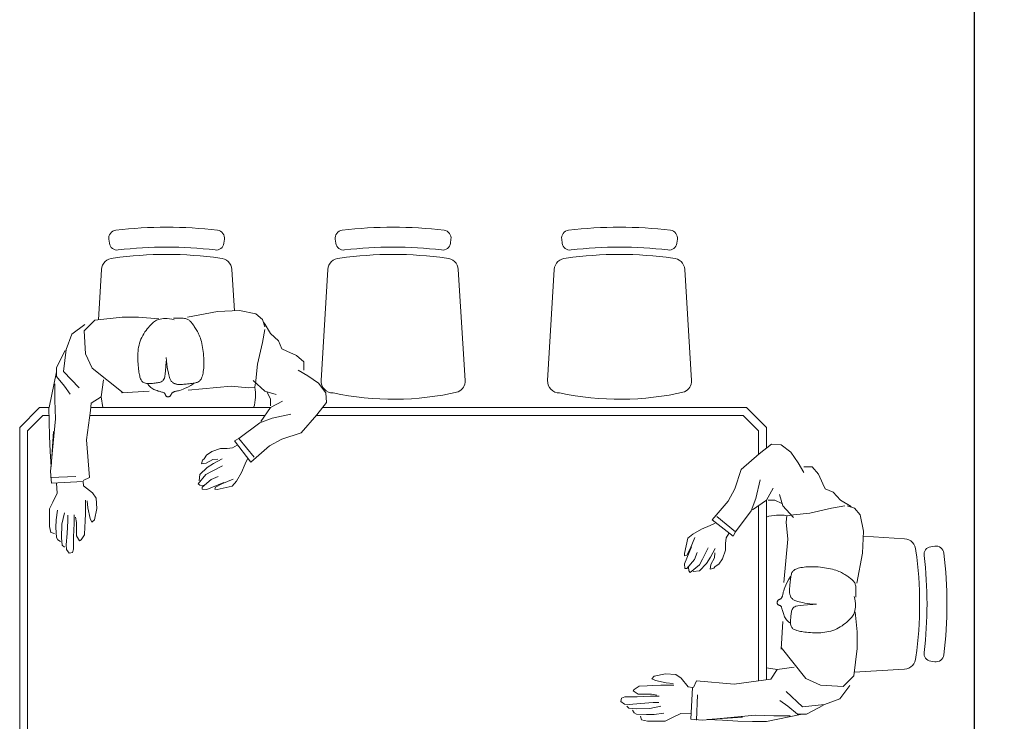
# Model space of a CAD drawing. Units: inches. Extents: x 1566 to 2546, y 1087 to 2705.
# Tile 9 of 27: x 1675 to 1773, y 1574 to 1643. Entities that reach past the tile are written whole.
import ezdxf

# ---------------------------------------------------------------- set-up
doc = ezdxf.new("R2010")
doc.units = ezdxf.units.IN
doc.layers.add('A-ANNO-DIMS', color=2, linetype='Continuous', lineweight=18)
doc.layers.add('A-FURN', color=8, linetype='Continuous', lineweight=18)
doc.styles.get("Standard").update_dxf_attribs({"font": 'arial.ttf'})
doc.dimstyles.new('ISO-25', dxfattribs={"dimtxt": 2.5, "dimasz": 2.5, "dimexe": 1.25, "dimexo": 0.625, "dimtad": 1, "dimtxsty": 'Standard', "dimcen": 2.5, "dimadec": 0, "dimazin": 0, "dimtfac": 1, "dimtmove": 0, "dimatfit": 3, "dimfxl": 1, "dimarcsym": 0})

# ---------------------------------------------------------------- blocks, each defined once
blk = doc.blocks.new('A$C421907B3')
for p, q in [((0.7079, 2.565), (0.7245, 2.5796)), ((0.7245, 2.5796), (0.7652, 2.5876)), ((0.7652, 2.5876), (0.8209, 2.5856)), ((0.8209, 2.5856), (0.8965, 2.5714)), ((0.7038, 2.5568), (0.6875, 2.5302)), ((0.7017, 2.5468), (0.7079, 2.565)), ((0.8839, 2.5541), (0.8823, 2.5521)), ((0.8853, 2.556), (0.8839, 2.5541)), ((0.8868, 2.5577), (0.8853, 2.556)), ((0.8883, 2.5594), (0.8868, 2.5577)), ((0.8897, 2.5609), (0.8883, 2.5594)), ((0.8911, 2.5623), (0.8897, 2.5609)), ((0.8926, 2.5635), (0.8911, 2.5623)), ((0.8941, 2.5647), (0.8926, 2.5635)), ((0.8958, 2.5657), (0.8941, 2.5647)), ((0.8976, 2.5665), (0.8958, 2.5657)), ((0.8996, 2.5672), (0.8976, 2.5665)), ((0.9018, 2.5678), (0.8996, 2.5672)), ((0.9043, 2.5682), (0.9018, 2.5678)), ((0.9071, 2.5684), (0.9043, 2.5682)), ((0.9102, 2.5686), (0.9071, 2.5684)), ((0.9137, 2.5687), (0.9102, 2.5686)), ((0.9175, 2.5687), (0.9137, 2.5687)), ((0.9217, 2.5687), (0.9175, 2.5687)), ((0.9264, 2.5687), (0.9217, 2.5687)), ((0.9314, 2.5687), (0.9264, 2.5687)), ((0.9361, 2.5662), (0.9297, 2.5647)), ((0.942, 2.5671), (0.9361, 2.5662)), ((0.9475, 2.5676), (0.942, 2.5671)), ((0.9525, 2.5677), (0.9475, 2.5676)), ((0.9571, 2.5675), (0.9525, 2.5677)), ((0.9614, 2.5669), (0.9571, 2.5675)), ((0.9652, 2.5662), (0.9614, 2.5669)), ((0.9686, 2.5653), (0.9652, 2.5662)), ((0.9684, 2.5672), (1.0195, 2.5715)), ((0.9717, 2.5643), (0.9686, 2.5653)), ((0.9745, 2.5632), (0.9717, 2.5643)), ((0.977, 2.5619), (0.9745, 2.5632)), ((0.9794, 2.5605), (0.977, 2.5619)), ((0.9818, 2.5588), (0.9794, 2.5605)), ((0.9841, 2.5568), (0.9818, 2.5588)), ((0.9865, 2.5545), (0.9841, 2.5568)), ((0.9891, 2.5519), (0.9865, 2.5545)), ((1.0195, 2.5715), (1.0607, 2.5715)), ((1.0607, 2.5715), (1.1301, 2.5633)), ((1.1301, 2.5633), (1.1567, 2.5368)), ((0.6875, 2.5302), (0.6672, 2.5117)), ((0.7017, 2.5405), (0.7079, 2.5077)), ((0.8684, 2.5289), (0.8669, 2.5256)), ((0.8699, 2.5321), (0.8684, 2.5289)), ((0.8714, 2.5351), (0.8699, 2.5321)), ((0.873, 2.5379), (0.8714, 2.5351)), ((0.8745, 2.5405), (0.873, 2.5379)), ((0.8761, 2.543), (0.8745, 2.5405)), ((0.8777, 2.5455), (0.8761, 2.543)), ((0.8792, 2.5478), (0.8777, 2.5455)), ((0.8808, 2.55), (0.8792, 2.5478)), ((0.8823, 2.5521), (0.8808, 2.55)), ((0.9918, 2.5489), (0.9891, 2.5519)), ((0.9948, 2.5455), (0.9918, 2.5489)), ((0.9978, 2.5419), (0.9948, 2.5455)), ((1.0008, 2.5379), (0.9978, 2.5419)), ((1.0037, 2.5338), (1.0008, 2.5379)), ((1.0066, 2.5294), (1.0037, 2.5338)), ((1.0093, 2.5249), (1.0066, 2.5294)), ((1.1567, 2.5368), (1.153, 2.4792)), ((1.1546, 2.5531), (1.1875, 2.5285)), ((1.1875, 2.5285), (1.202, 2.4895)), ((0.6672, 2.5117), (0.6589, 2.4912)), ((0.7079, 2.5077), (0.7204, 2.4524)), ((0.8604, 2.5049), (0.8594, 2.5001)), ((0.8616, 2.5096), (0.8604, 2.5049)), ((0.8628, 2.514), (0.8616, 2.5096)), ((0.8641, 2.5181), (0.8628, 2.514)), ((0.8655, 2.522), (0.8641, 2.5181)), ((0.8669, 2.5256), (0.8655, 2.522)), ((1.0117, 2.5203), (1.0093, 2.5249)), ((1.0138, 2.5155), (1.0117, 2.5203)), ((1.0156, 2.5107), (1.0138, 2.5155)), ((1.0171, 2.5058), (1.0156, 2.5107)), ((1.0184, 2.5008), (1.0171, 2.5058)), ((0.6464, 2.4852), (0.6219, 2.4749)), ((0.6589, 2.4912), (0.6464, 2.4852)), ((0.8562, 2.4794), (0.8558, 2.474)), ((0.8568, 2.4847), (0.8562, 2.4794)), ((0.8576, 2.49), (0.8568, 2.4847)), ((0.8584, 2.4951), (0.8576, 2.49)), ((0.8594, 2.5001), (0.8584, 2.4951)), ((1.0194, 2.4958), (1.0184, 2.5008)), ((1.0202, 2.4907), (1.0194, 2.4958)), ((1.0208, 2.4855), (1.0202, 2.4907)), ((1.0212, 2.4802), (1.0208, 2.4855)), ((1.0214, 2.4749), (1.0212, 2.4802)), ((1.153, 2.4792), (1.1364, 2.4424)), ((1.202, 2.4895), (1.2083, 2.4342)), ((1.2041, 2.4875), (1.2266, 2.4445)), ((0.6219, 2.4749), (0.6036, 2.4584)), ((0.6036, 2.4584), (0.6036, 2.4379)), ((0.8552, 2.4632), (0.8551, 2.4579)), ((0.8551, 2.4579), (0.8552, 2.4527)), ((0.8554, 2.4686), (0.8552, 2.4632)), ((0.8558, 2.474), (0.8554, 2.4686)), ((0.9483, 2.453), (0.9491, 2.4609)), ((0.9491, 2.4609), (0.9498, 2.4698)), ((0.9505, 2.4603), (0.9511, 2.447)), ((1.021, 2.4541), (1.0212, 2.4591)), ((1.0212, 2.4591), (1.0214, 2.4643)), ((1.0215, 2.4696), (1.0214, 2.4749)), ((1.0214, 2.4643), (1.0215, 2.4696)), ((0.6178, 2.4379), (0.5933, 2.4236)), ((0.7204, 2.4524), (0.7246, 2.4114)), ((0.8552, 2.4527), (0.8554, 2.4476)), ((0.8554, 2.4476), (0.8557, 2.4428)), ((0.8557, 2.4428), (0.8561, 2.4383)), ((0.8561, 2.4383), (0.8567, 2.4341)), ((0.8567, 2.4341), (0.8574, 2.4301)), ((0.8574, 2.4301), (0.8582, 2.4265)), ((0.9435, 2.426), (0.9445, 2.43)), ((0.9445, 2.43), (0.9455, 2.4346)), ((0.9455, 2.4346), (0.9465, 2.4399)), ((0.9465, 2.4399), (0.9474, 2.446)), ((0.9474, 2.446), (0.9483, 2.453)), ((0.9511, 2.447), (0.9518, 2.4364)), ((0.9518, 2.4364), (0.9526, 2.4283)), ((1.0181, 2.429), (1.0186, 2.4325)), ((1.0186, 2.4325), (1.0192, 2.4362)), ((1.0192, 2.4362), (1.0197, 2.4402)), ((1.0197, 2.4402), (1.0202, 2.4445)), ((1.0202, 2.4445), (1.0206, 2.4492)), ((1.0206, 2.4492), (1.021, 2.4541)), ((1.1364, 2.4424), (1.0587, 2.3808)), ((1.2083, 2.4342), (1.1693, 2.3932)), ((1.2266, 2.4445), (1.2266, 2.422)), ((1.2447, 2.3435), (1.2266, 2.4332)), ((0.5667, 2.4051), (0.5484, 2.3805)), ((0.5933, 2.4236), (0.5667, 2.4051)), ((0.7308, 2.4114), (0.7018, 2.3846)), ((0.7246, 2.4114), (0.7267, 2.3949)), ((0.8582, 2.4265), (0.8591, 2.4232)), ((0.8591, 2.4232), (0.8601, 2.4202)), ((0.8601, 2.4202), (0.8612, 2.4176)), ((0.8612, 2.4176), (0.8624, 2.4152)), ((0.8624, 2.4152), (0.8637, 2.4132)), ((0.8637, 2.4132), (0.8651, 2.4114)), ((0.8651, 2.4114), (0.8666, 2.41)), ((0.8666, 2.41), (0.8682, 2.4088)), ((0.8682, 2.4088), (0.87, 2.4078)), ((0.87, 2.4078), (0.872, 2.407)), ((0.872, 2.407), (0.8742, 2.4063)), ((0.8742, 2.4063), (0.8767, 2.4058)), ((0.8767, 2.4058), (0.8794, 2.4052)), ((0.8794, 2.4052), (0.8824, 2.4048)), ((0.8824, 2.4048), (0.8857, 2.4043)), ((0.9301, 2.4044), (0.9315, 2.4052)), ((0.9315, 2.4052), (0.9329, 2.406)), ((0.9329, 2.406), (0.9341, 2.4069)), ((0.9341, 2.4069), (0.9353, 2.4079)), ((0.9353, 2.4079), (0.9363, 2.409)), ((0.9363, 2.409), (0.9373, 2.4102)), ((0.9373, 2.4102), (0.9382, 2.4116)), ((0.9382, 2.4116), (0.9391, 2.4131)), ((0.9391, 2.4131), (0.9399, 2.415)), ((0.9399, 2.415), (0.9408, 2.4171)), ((0.9408, 2.4171), (0.9416, 2.4196)), ((0.9416, 2.4196), (0.9425, 2.4226)), ((0.9425, 2.4226), (0.9435, 2.426)), ((0.9526, 2.4283), (0.9535, 2.4222)), ((0.9535, 2.4222), (0.9546, 2.4177)), ((0.9546, 2.4177), (0.9558, 2.4146)), ((0.9558, 2.4146), (0.9572, 2.4124)), ((0.9572, 2.4124), (0.9588, 2.4109)), ((0.9588, 2.4109), (0.9606, 2.4096)), ((0.9606, 2.4096), (0.9626, 2.4086)), ((0.9626, 2.4086), (0.9647, 2.4077)), ((0.9647, 2.4077), (0.9671, 2.407)), ((0.9671, 2.407), (0.9696, 2.4064)), ((0.9696, 2.4064), (0.9722, 2.406)), ((0.9722, 2.406), (0.9751, 2.4055)), ((0.9751, 2.4055), (0.9781, 2.4052)), ((0.9781, 2.4052), (0.9812, 2.4048)), ((0.9812, 2.4048), (0.9844, 2.4045)), ((0.9844, 2.4045), (0.9877, 2.4043)), ((0.9999, 2.4044), (1.0025, 2.4049)), ((1.0025, 2.4049), (1.0047, 2.4055)), ((1.0047, 2.4055), (1.0067, 2.4064)), ((1.0067, 2.4064), (1.0085, 2.4075)), ((1.0085, 2.4075), (1.01, 2.4087)), ((1.01, 2.4087), (1.0113, 2.4102)), ((1.0113, 2.4102), (1.0124, 2.4119)), ((1.0124, 2.4119), (1.0135, 2.4137)), ((1.0135, 2.4137), (1.0144, 2.4158)), ((1.0144, 2.4158), (1.0152, 2.418)), ((1.0152, 2.418), (1.016, 2.4204)), ((1.016, 2.4204), (1.0168, 2.423)), ((1.0168, 2.423), (1.0174, 2.4259)), ((1.0174, 2.4259), (1.0181, 2.429)), ((1.1077, 2.4136), (1.114, 2.3706)), ((1.2266, 2.422), (1.2062, 2.3974)), ((0.5484, 2.3805), (0.5463, 2.356)), ((0.7018, 2.3846), (0.6731, 2.3766)), ((0.6876, 2.3643), (0.6959, 2.3826)), ((0.7267, 2.3949), (0.7429, 2.3929)), ((0.7429, 2.3929), (0.7861, 2.3972)), ((0.7861, 2.3972), (0.8946, 2.387)), ((0.8801, 2.4042), (0.8884, 2.3992)), ((0.8857, 2.4043), (0.8891, 2.4039)), ((0.8884, 2.3992), (0.8957, 2.3952)), ((0.8891, 2.4039), (0.8925, 2.4035)), ((0.8925, 2.4035), (0.896, 2.4031)), ((0.8957, 2.3952), (0.9019, 2.3921)), ((0.896, 2.4031), (0.8995, 2.4027)), ((0.8995, 2.4027), (0.9028, 2.4024)), ((0.9019, 2.3921), (0.9073, 2.3897)), ((0.9028, 2.4024), (0.9059, 2.4022)), ((0.9059, 2.4022), (0.9088, 2.4019)), ((0.9073, 2.3897), (0.9119, 2.3881)), ((0.9088, 2.4019), (0.9114, 2.4018)), ((0.9114, 2.4018), (0.9138, 2.4016)), ((0.9119, 2.3881), (0.9157, 2.3869)), ((0.9138, 2.4016), (0.9161, 2.4016)), ((0.9157, 2.3869), (0.919, 2.386)), ((0.9161, 2.4016), (0.9182, 2.4016)), ((0.9182, 2.4016), (0.9201, 2.4017)), ((0.919, 2.386), (0.9217, 2.3854)), ((0.9201, 2.4017), (0.9219, 2.4019)), ((0.9217, 2.3854), (0.924, 2.3849)), ((0.9219, 2.4019), (0.9237, 2.4022)), ((0.9237, 2.4022), (0.9254, 2.4026)), ((0.924, 2.3849), (0.926, 2.3844)), ((0.9254, 2.4026), (0.927, 2.4031)), ((0.926, 2.3844), (0.9277, 2.384)), ((0.927, 2.4031), (0.9286, 2.4037)), ((0.9277, 2.384), (0.929, 2.3837)), ((0.9286, 2.4037), (0.9301, 2.4044)), ((0.929, 2.3837), (0.9302, 2.3833)), ((0.9302, 2.3833), (0.9312, 2.383)), ((0.9312, 2.383), (0.932, 2.3826)), ((0.932, 2.3826), (0.9327, 2.3823)), ((0.9327, 2.3823), (0.9334, 2.3818)), ((0.9334, 2.3818), (0.934, 2.3813)), ((0.934, 2.3813), (0.9346, 2.3808)), ((0.9346, 2.3808), (0.9351, 2.3803)), ((0.9351, 2.3803), (0.9356, 2.3797)), ((0.954, 2.3796), (0.9546, 2.3801)), ((0.9546, 2.3801), (0.9554, 2.3805)), ((0.9554, 2.3805), (0.9564, 2.381)), ((0.9564, 2.381), (0.9577, 2.3815)), ((0.9577, 2.3815), (0.9593, 2.382)), ((0.9593, 2.382), (0.9611, 2.3826)), ((0.9611, 2.3826), (0.9632, 2.3832)), ((0.9632, 2.3832), (0.9655, 2.3838)), ((0.9655, 2.3838), (0.9679, 2.3845)), ((0.9679, 2.3845), (0.9705, 2.3853)), ((0.9705, 2.3853), (0.9731, 2.3861)), ((0.9731, 2.3861), (0.9757, 2.387)), ((0.9757, 2.387), (0.9784, 2.388)), ((0.9784, 2.388), (0.9811, 2.3892)), ((0.9811, 2.3892), (0.9837, 2.3905)), ((0.9837, 2.3905), (0.9863, 2.3922)), ((0.9863, 2.3922), (0.9889, 2.3941)), ((0.9877, 2.4043), (0.9909, 2.4041)), ((0.9889, 2.3941), (0.9915, 2.3965)), ((0.9909, 2.4041), (0.9941, 2.4041)), ((0.9915, 2.3965), (0.994, 2.3993)), ((0.9931, 2.3848), (1.0625, 2.3808)), ((0.994, 2.3993), (0.9965, 2.4026)), ((0.9941, 2.4041), (0.9971, 2.4042)), ((0.9971, 2.4042), (0.9999, 2.4044)), ((1.2062, 2.3974), (1.1917, 2.3769)), ((1.2308, 2.3624), (1.2308, 2.4035)), ((0.5463, 2.356), (0.5709, 2.3252)), ((0.6569, 2.3601), (0.6876, 2.3438)), ((0.6876, 2.3478), (0.6876, 2.3643)), ((0.9356, 2.3797), (0.936, 2.379)), ((0.936, 2.379), (0.9365, 2.3783)), ((0.9365, 2.3783), (0.9369, 2.3776)), ((0.9369, 2.3776), (0.9372, 2.3769)), ((0.9372, 2.3769), (0.9376, 2.3761)), ((0.9376, 2.3761), (0.938, 2.3753)), ((0.938, 2.3753), (0.9384, 2.3746)), ((0.9384, 2.3746), (0.9389, 2.3738)), ((0.9389, 2.3738), (0.9395, 2.3731)), ((0.9395, 2.3731), (0.9401, 2.3725)), ((0.9401, 2.3725), (0.9408, 2.3719)), ((0.9408, 2.3719), (0.9417, 2.3714)), ((0.9417, 2.3714), (0.9426, 2.371)), ((0.9426, 2.371), (0.9437, 2.3707)), ((0.9437, 2.3707), (0.9447, 2.3706)), ((0.9447, 2.3706), (0.9458, 2.3705)), ((0.9458, 2.3705), (0.9468, 2.3706)), ((0.9468, 2.3706), (0.9478, 2.3708)), ((0.9478, 2.3708), (0.9487, 2.3712)), ((0.9487, 2.3712), (0.9494, 2.3717)), ((0.9494, 2.3717), (0.9501, 2.3723)), ((0.9501, 2.3723), (0.9507, 2.3731)), ((0.9507, 2.3731), (0.9512, 2.3739)), ((0.9512, 2.3739), (0.9517, 2.3747)), ((0.9517, 2.3747), (0.9521, 2.3755)), ((0.9521, 2.3755), (0.9524, 2.3764)), ((0.9524, 2.3764), (0.9527, 2.3771)), ((0.9527, 2.3771), (0.953, 2.3778)), ((0.953, 2.3778), (0.9533, 2.3785)), ((0.9533, 2.3785), (0.9536, 2.379)), ((0.9536, 2.379), (0.954, 2.3796)), ((1.114, 2.3706), (1.1095, 2.3436)), ((1.114, 2.3706), (1.1385, 2.3544)), ((1.2287, 2.3154), (1.2308, 2.3624)), ((0.6876, 2.3438), (0.7122, 2.3088)), ((1.1385, 2.3544), (1.1406, 2.3358)), ((1.1406, 2.3358), (1.151, 2.262)), ((0.5709, 2.3252), (0.6099, 2.2802)), ((0.6835, 2.317), (0.6365, 2.3273)), ((0.7143, 2.3048), (0.6835, 2.317)), ((1.235, 2.2538), (1.2287, 2.3154)), ((0.7674, 2.2656), (0.7143, 2.3048)), ((0.6099, 2.2802), (0.659, 2.2637)), ((0.659, 2.2637), (0.6898, 2.2475)), ((0.7288, 2.2187), (0.7675, 2.2658)), ((0.7779, 2.2598), (0.7368, 2.2065)), ((0.7675, 2.2658), (0.7779, 2.2598)), ((1.151, 2.262), (1.1428, 2.1677)), ((0.6898, 2.2475), (0.7368, 2.2065)), ((0.7716, 2.2487), (0.7827, 2.2421)), ((0.7827, 2.2421), (0.7969, 2.2406)), ((0.7969, 2.2406), (0.8131, 2.2406)), ((0.8131, 2.2406), (0.8354, 2.2325)), ((0.8354, 2.2325), (0.8487, 2.2236)), ((1.2413, 2.1822), (1.235, 2.2538)), ((0.7509, 2.2021), (0.7458, 2.2146)), ((0.8094, 2.2146), (0.8309, 2.2028)), ((0.8324, 2.2124), (0.8198, 2.2132)), ((0.8494, 2.2036), (0.8324, 2.2124)), ((0.8487, 2.2236), (0.8546, 2.2147)), ((0.8546, 2.2147), (0.859, 2.211)), ((0.859, 2.211), (0.8613, 2.2021)), ((0.7606, 2.1798), (0.7509, 2.2021)), ((0.8079, 2.1969), (0.8361, 2.1828)), ((0.8309, 2.2028), (0.8472, 2.1925)), ((0.8361, 2.1828), (0.8502, 2.1747)), ((0.8472, 2.1925), (0.8658, 2.1747)), ((0.8613, 2.2021), (0.8494, 2.2036)), ((1.2392, 2.1535), (1.2413, 2.1822)), ((0.7732, 2.1583), (0.7606, 2.1798)), ((0.7835, 2.1457), (0.7732, 2.1583)), ((0.7814, 2.1628), (0.8102, 2.1517)), ((0.8191, 2.1695), (0.8369, 2.1621)), ((0.8369, 2.1621), (0.8599, 2.1429)), ((0.8502, 2.1747), (0.8695, 2.1518)), ((0.8658, 2.1747), (0.8672, 2.1591)), ((1.1428, 2.1677), (1.159, 2.1597)), ((1.1595, 2.1573), (1.158, 2.1467)), ((1.1595, 2.1573), (1.2392, 2.1535)), ((1.1777, 2.1697), (1.2413, 2.1677)), ((0.8221, 2.1369), (0.7835, 2.1457)), ((0.848, 2.1369), (0.805, 2.1547)), ((0.8102, 2.1517), (0.8257, 2.1428)), ((0.828, 2.1376), (0.8221, 2.1369)), ((0.8257, 2.1428), (0.828, 2.1376)), ((0.8599, 2.1384), (0.848, 2.1369)), ((0.8658, 2.1481), (0.8561, 2.1473)), ((0.8599, 2.1429), (0.8599, 2.1384)), ((0.8695, 2.1518), (0.8658, 2.1481)), ((1.158, 2.1467), (1.1354, 2.1286)), ((1.226, 2.1528), (1.2245, 2.1279)), ((1.1263, 2.1158), (1.1248, 2.0893)), ((1.1354, 2.1286), (1.1263, 2.1158)), ((1.1474, 2.0909), (1.149, 2.1089)), ((1.1535, 2.1105), (1.1536, 2.078)), ((1.2245, 2.1279), (1.2358, 2.1052)), ((1.1248, 2.0893), (1.1308, 2.0606)), ((1.1414, 2.0644), (1.1474, 2.0909)), ((1.2238, 2.0848), (1.2269, 2.0606)), ((1.2358, 2.1052), (1.2442, 2.0886)), ((1.2442, 2.0886), (1.2442, 2.0441)), ((1.1308, 2.0606), (1.1377, 2.0553)), ((1.1377, 2.0553), (1.1414, 2.0644)), ((1.1536, 2.078), (1.1543, 2.0568)), ((1.1762, 2.0539), (1.1784, 2.0674)), ((1.1815, 2.0735), (1.1815, 2.0516)), ((1.1974, 2.0584), (1.1974, 2.0727)), ((1.1996, 2.0267), (1.1974, 2.0584)), ((1.2064, 2.078), (1.2125, 2.0501)), ((1.2269, 2.0606), (1.2276, 2.0418)), ((1.1543, 2.0568), (1.1551, 2.0432)), ((1.1551, 2.0432), (1.1558, 2.0229)), ((1.1762, 2.0357), (1.1762, 2.0539)), ((1.1762, 2.0206), (1.1762, 2.0357)), ((1.1815, 2.0516), (1.1831, 2.0183)), ((1.2125, 2.0501), (1.2132, 2.0154)), ((1.2276, 2.0418), (1.2261, 2.0161)), ((1.2442, 2.0441), (1.2404, 2.029)), ((1.1558, 2.0229), (1.1641, 2.0108)), ((1.1641, 2.0108), (1.168, 2.0077)), ((1.168, 2.0077), (1.1762, 2.0206)), ((1.1831, 2.0183), (1.1831, 1.9874)), ((1.2019, 1.9979), (1.1996, 2.0267)), ((1.2132, 2.0154), (1.2117, 1.9972)), ((1.223, 2.0108), (1.2163, 2.0063)), ((1.2261, 2.0161), (1.223, 2.0108)), ((1.2404, 2.029), (1.2314, 2.0267)), ((1.1831, 1.9874), (1.186, 1.9783)), ((1.1944, 1.9768), (1.2012, 1.9859)), ((1.2012, 1.9859), (1.2019, 1.9979)), ((1.2117, 1.9972), (1.2064, 1.9919)), ((1.186, 1.9783), (1.1944, 1.9768)), ((0.3742, 1.1891), (0.3928, 1.2157)), ((0.3928, 1.2157), (0.4173, 1.234)), ((0.4173, 1.234), (0.4418, 1.2361)), ((0.4418, 1.2361), (0.4726, 1.2115)), ((0.4726, 1.2115), (0.5176, 1.1724)), ((0.3229, 1.1605), (0.3394, 1.1788)), ((0.3394, 1.1788), (0.36, 1.1787)), ((0.36, 1.1646), (0.3742, 1.1891)), ((0.5176, 1.1724), (0.5341, 1.1234)), ((0.3126, 1.1359), (0.3229, 1.1605)), ((0.4808, 1.0989), (0.4706, 1.1459)), ((0.2861, 1.1152), (0.3066, 1.1235)), ((0.3066, 1.1235), (0.3126, 1.1359)), ((0.4378, 1.1255), (0.454, 1.0947)), ((0.5341, 1.1234), (0.5503, 1.0926)), ((0.241, 1.0786), (0.2676, 1.0948)), ((0.2676, 1.0948), (0.2861, 1.1152)), ((0.4132, 1.0806), (0.4212, 1.1093)), ((0.4335, 1.0947), (0.4152, 1.0865)), ((0.45, 1.0947), (0.4335, 1.0947)), ((0.454, 1.0947), (0.489, 1.0702)), ((0.493, 1.0681), (0.4808, 1.0989)), ((0.5503, 1.0926), (0.5914, 1.0456)), ((0.2328, 1.0745), (0.2183, 1.0579)), ((0.2511, 1.0807), (0.2328, 1.0745)), ((0.2573, 1.0807), (0.2901, 1.0744)), ((0.2901, 1.0744), (0.3454, 1.062)), ((0.3864, 1.0516), (0.4132, 1.0806)), ((0.5322, 1.015), (0.493, 1.0681)), ((0.2183, 1.0579), (0.2102, 1.0171)), ((0.3454, 1.062), (0.3864, 1.0578)), ((0.3864, 1.0578), (0.4029, 1.0557)), ((0.4029, 1.0557), (0.4049, 1.0395)), ((0.5791, 1.0535), (0.532, 1.0149)), ((0.538, 1.0045), (0.5914, 1.0456)), ((0.2102, 1.0171), (0.2122, 0.9615)), ((0.4049, 1.0395), (0.4006, 0.9963)), ((0.5958, 1.0315), (0.5832, 1.0366)), ((0.618, 1.0218), (0.5958, 1.0315)), ((0.6395, 1.0092), (0.618, 1.0218)), ((0.4006, 0.9963), (0.4108, 0.8878)), ((0.532, 1.0149), (0.538, 1.0045)), ((0.5491, 1.0108), (0.5557, 0.9996)), ((0.5557, 0.9996), (0.5572, 0.9855)), ((0.635, 1.001), (0.6461, 0.9722)), ((0.6521, 0.9988), (0.6395, 1.0092)), ((0.6609, 0.9603), (0.6521, 0.9988)), ((0.5572, 0.9855), (0.5572, 0.9693)), ((0.5572, 0.9693), (0.5653, 0.947)), ((0.5832, 0.9729), (0.595, 0.9515)), ((0.6009, 0.9744), (0.615, 0.9462)), ((0.6609, 0.9344), (0.6432, 0.9774)), ((0.6461, 0.9722), (0.655, 0.9566)), ((0.2122, 0.9615), (0.2264, 0.8858)), ((0.5653, 0.947), (0.5742, 0.9337)), ((0.5854, 0.9499), (0.5846, 0.9626)), ((0.5942, 0.933), (0.5854, 0.9499)), ((0.595, 0.9515), (0.6053, 0.9352)), ((0.615, 0.9462), (0.6232, 0.9322)), ((0.6283, 0.9633), (0.6357, 0.9455)), ((0.6357, 0.9455), (0.655, 0.9225)), ((0.655, 0.9566), (0.6602, 0.9544)), ((0.6602, 0.9544), (0.6609, 0.9603)), ((0.2759, 0.9169), (0.2797, 0.9183)), ((0.2797, 0.9183), (0.2839, 0.9196)), ((0.2839, 0.9196), (0.2883, 0.9208)), ((0.2883, 0.9208), (0.2929, 0.922)), ((0.2929, 0.922), (0.2977, 0.923)), ((0.2977, 0.923), (0.3027, 0.924)), ((0.3027, 0.924), (0.3078, 0.9248)), ((0.3078, 0.9248), (0.3131, 0.9255)), ((0.3131, 0.9255), (0.3184, 0.9261)), ((0.3184, 0.9261), (0.3238, 0.9266)), ((0.3238, 0.9266), (0.3293, 0.927)), ((0.3293, 0.927), (0.3347, 0.9272)), ((0.3347, 0.9272), (0.34, 0.9272)), ((0.34, 0.9272), (0.3452, 0.9272)), ((0.3452, 0.9272), (0.3502, 0.927)), ((0.3502, 0.927), (0.355, 0.9267)), ((0.355, 0.9267), (0.3595, 0.9262)), ((0.3595, 0.9262), (0.3638, 0.9257)), ((0.3638, 0.9257), (0.3677, 0.925)), ((0.3677, 0.925), (0.3713, 0.9242)), ((0.3713, 0.9242), (0.3746, 0.9233)), ((0.3746, 0.9233), (0.3776, 0.9223)), ((0.3776, 0.9223), (0.3803, 0.9212)), ((0.3803, 0.9212), (0.3826, 0.92)), ((0.3826, 0.92), (0.3847, 0.9187)), ((0.3847, 0.9187), (0.3864, 0.9173)), ((0.3864, 0.9173), (0.3878, 0.9158)), ((0.5742, 0.9337), (0.5832, 0.9278)), ((0.5832, 0.9278), (0.5869, 0.9233)), ((0.5869, 0.9233), (0.5957, 0.9211)), ((0.5957, 0.9211), (0.5942, 0.933)), ((0.6053, 0.9352), (0.6232, 0.9166)), ((0.6232, 0.9322), (0.6461, 0.9129)), ((0.6498, 0.9166), (0.6506, 0.9263)), ((0.655, 0.9225), (0.6594, 0.9225)), ((0.6594, 0.9225), (0.6609, 0.9344)), ((0.2356, 0.8913), (0.237, 0.8927)), ((0.237, 0.8927), (0.2385, 0.8941)), ((0.2385, 0.8941), (0.2401, 0.8956)), ((0.2401, 0.8956), (0.2419, 0.897)), ((0.2419, 0.897), (0.2437, 0.8985)), ((0.2437, 0.8985), (0.2457, 0.9)), ((0.2457, 0.9), (0.2478, 0.9016)), ((0.2478, 0.9016), (0.25, 0.9031)), ((0.25, 0.9031), (0.2524, 0.9047)), ((0.2524, 0.9047), (0.2548, 0.9063)), ((0.2548, 0.9063), (0.2573, 0.9078)), ((0.2573, 0.9078), (0.26, 0.9094)), ((0.26, 0.9094), (0.2628, 0.911)), ((0.2628, 0.911), (0.2657, 0.9125)), ((0.2657, 0.9125), (0.2689, 0.914)), ((0.2689, 0.914), (0.2723, 0.9155)), ((0.2723, 0.9155), (0.2759, 0.9169)), ((0.3878, 0.9158), (0.389, 0.9142)), ((0.389, 0.9142), (0.39, 0.9123)), ((0.39, 0.9123), (0.3908, 0.9104)), ((0.3908, 0.9104), (0.3915, 0.9081)), ((0.3915, 0.9081), (0.3921, 0.9057)), ((0.3921, 0.9057), (0.3926, 0.903)), ((0.3926, 0.903), (0.3931, 0.8999)), ((0.3931, 0.8999), (0.3935, 0.8967)), ((0.3935, 0.8967), (0.394, 0.8933)), ((0.3936, 0.9023), (0.3986, 0.894)), ((0.394, 0.8933), (0.3944, 0.8898)), ((0.3986, 0.894), (0.4026, 0.8867)), ((0.6232, 0.9166), (0.6387, 0.9151)), ((0.6461, 0.9129), (0.6498, 0.9166)), ((0.2291, 0.8687), (0.2292, 0.8722)), ((0.2291, 0.8649), (0.2291, 0.8687)), ((0.2292, 0.8722), (0.2294, 0.8753)), ((0.2294, 0.8753), (0.2297, 0.8781)), ((0.2297, 0.8781), (0.2301, 0.8806)), ((0.2301, 0.8806), (0.2306, 0.8828)), ((0.2306, 0.8828), (0.2313, 0.8848)), ((0.2313, 0.8848), (0.2322, 0.8866)), ((0.2322, 0.8866), (0.2332, 0.8883)), ((0.2332, 0.8883), (0.2343, 0.8898)), ((0.2343, 0.8898), (0.2356, 0.8913)), ((0.3944, 0.8898), (0.3947, 0.8863)), ((0.3947, 0.8863), (0.3951, 0.8829)), ((0.3951, 0.8829), (0.3954, 0.8796)), ((0.3954, 0.8796), (0.3957, 0.8765)), ((0.3957, 0.8765), (0.3959, 0.8736)), ((0.3959, 0.8736), (0.3961, 0.871)), ((0.3961, 0.871), (0.3962, 0.8685)), ((0.3962, 0.8685), (0.3962, 0.8663)), ((0.4026, 0.8867), (0.4057, 0.8804)), ((0.4057, 0.8804), (0.4081, 0.8751)), ((0.4081, 0.8751), (0.4098, 0.8705)), ((0.4098, 0.8705), (0.411, 0.8667)), ((0.2291, 0.8607), (0.2291, 0.8649)), ((0.2291, 0.856), (0.2291, 0.8607)), ((0.2291, 0.8509), (0.2291, 0.856)), ((0.2307, 0.8404), (0.2316, 0.8463)), ((0.2316, 0.8463), (0.2331, 0.8527)), ((0.3847, 0.8433), (0.3829, 0.8425)), ((0.3863, 0.8442), (0.3847, 0.8433)), ((0.3876, 0.8451), (0.3863, 0.8442)), ((0.3888, 0.846), (0.3876, 0.8451)), ((0.3899, 0.8471), (0.3888, 0.846)), ((0.3909, 0.8482), (0.3899, 0.8471)), ((0.3918, 0.8495), (0.3909, 0.8482)), ((0.3927, 0.8508), (0.3918, 0.8495)), ((0.3934, 0.8523), (0.3927, 0.8508)), ((0.3941, 0.8538), (0.3934, 0.8523)), ((0.3947, 0.8553), (0.3941, 0.8538)), ((0.3952, 0.857), (0.3947, 0.8553)), ((0.3956, 0.8587), (0.3952, 0.857)), ((0.3959, 0.8604), (0.3956, 0.8587)), ((0.3961, 0.8623), (0.3959, 0.8604)), ((0.3962, 0.8642), (0.3961, 0.8623)), ((0.3962, 0.8663), (0.3962, 0.8642)), ((0.411, 0.8667), (0.4118, 0.8634)), ((0.4118, 0.8634), (0.4124, 0.8607)), ((0.4124, 0.8607), (0.4129, 0.8583)), ((0.4129, 0.8583), (0.4134, 0.8564)), ((0.4134, 0.8564), (0.4138, 0.8547)), ((0.4138, 0.8547), (0.4141, 0.8533)), ((0.4141, 0.8533), (0.4145, 0.8522)), ((0.4145, 0.8522), (0.4148, 0.8512)), ((0.4148, 0.8512), (0.4152, 0.8504)), ((0.4152, 0.8504), (0.4156, 0.8497)), ((0.4156, 0.8497), (0.416, 0.849)), ((0.416, 0.849), (0.4165, 0.8484)), ((0.4165, 0.8484), (0.417, 0.8478)), ((0.417, 0.8478), (0.4176, 0.8473)), ((0.4176, 0.8473), (0.4182, 0.8468)), ((0.4182, 0.8468), (0.4188, 0.8463)), ((0.4188, 0.8463), (0.4195, 0.8459)), ((0.4195, 0.8459), (0.4202, 0.8455)), ((0.4202, 0.8455), (0.4209, 0.8451)), ((0.4209, 0.8451), (0.4217, 0.8448)), ((0.4217, 0.8448), (0.4225, 0.8444)), ((0.4225, 0.8444), (0.4233, 0.8439)), ((0.4233, 0.8439), (0.424, 0.8435)), ((0.424, 0.8435), (0.4247, 0.8429)), ((0.4247, 0.8429), (0.4253, 0.8423)), ((0.2301, 0.8299), (0.2302, 0.8349)), ((0.2304, 0.8252), (0.2301, 0.8299)), ((0.2302, 0.8349), (0.2307, 0.8404)), ((0.2309, 0.821), (0.2304, 0.8252)), ((0.2316, 0.8172), (0.2309, 0.821)), ((0.3369, 0.8333), (0.328, 0.8326)), ((0.3448, 0.8341), (0.3369, 0.8333)), ((0.3375, 0.8319), (0.3508, 0.8313)), ((0.3518, 0.835), (0.3448, 0.8341)), ((0.3508, 0.8313), (0.3614, 0.8306)), ((0.3579, 0.8359), (0.3518, 0.835)), ((0.3632, 0.8369), (0.3579, 0.8359)), ((0.3614, 0.8306), (0.3695, 0.8298)), ((0.3678, 0.8379), (0.3632, 0.8369)), ((0.3718, 0.8389), (0.3678, 0.8379)), ((0.3695, 0.8298), (0.3757, 0.8289)), ((0.3752, 0.8398), (0.3718, 0.8389)), ((0.3782, 0.8407), (0.3752, 0.8398)), ((0.3757, 0.8289), (0.3801, 0.8278)), ((0.3807, 0.8416), (0.3782, 0.8407)), ((0.3801, 0.8278), (0.3832, 0.8265)), ((0.3829, 0.8425), (0.3807, 0.8416)), ((0.3832, 0.8265), (0.3854, 0.8251)), ((0.3854, 0.8251), (0.3869, 0.8235)), ((0.3869, 0.8235), (0.3882, 0.8218)), ((0.3882, 0.8218), (0.3892, 0.8198)), ((0.3892, 0.8198), (0.3901, 0.8176)), ((0.4147, 0.8192), (0.414, 0.8169)), ((0.4152, 0.8213), (0.4147, 0.8192)), ((0.4158, 0.8231), (0.4152, 0.8213)), ((0.4163, 0.8247), (0.4158, 0.8231)), ((0.4168, 0.826), (0.4163, 0.8247)), ((0.4173, 0.827), (0.4168, 0.826)), ((0.4178, 0.8277), (0.4173, 0.827)), ((0.4183, 0.8283), (0.4178, 0.8277)), ((0.4188, 0.8288), (0.4183, 0.8283)), ((0.4194, 0.8291), (0.4188, 0.8288)), ((0.42, 0.8294), (0.4194, 0.8291)), ((0.4207, 0.8297), (0.42, 0.8294)), ((0.4215, 0.83), (0.4207, 0.8297)), ((0.4223, 0.8303), (0.4215, 0.83)), ((0.4231, 0.8307), (0.4223, 0.8303)), ((0.424, 0.8311), (0.4231, 0.8307)), ((0.4248, 0.8316), (0.424, 0.8311)), ((0.4255, 0.8322), (0.4248, 0.8316)), ((0.4253, 0.8423), (0.4259, 0.8415)), ((0.4261, 0.8329), (0.4255, 0.8322)), ((0.4259, 0.8415), (0.4264, 0.8407)), ((0.4267, 0.8337), (0.4261, 0.8329)), ((0.4264, 0.8407), (0.4268, 0.8397)), ((0.427, 0.8346), (0.4267, 0.8337)), ((0.4268, 0.8397), (0.4271, 0.8387)), ((0.4272, 0.8356), (0.427, 0.8346)), ((0.4271, 0.8387), (0.4273, 0.8377)), ((0.4273, 0.8366), (0.4272, 0.8356)), ((0.4273, 0.8377), (0.4273, 0.8366)), ((0.2306, 0.814), (0.2263, 0.7628)), ((0.2325, 0.8138), (0.2316, 0.8172)), ((0.2335, 0.8107), (0.2325, 0.8138)), ((0.2346, 0.8079), (0.2335, 0.8107)), ((0.2359, 0.8053), (0.2346, 0.8079)), ((0.2374, 0.8029), (0.2359, 0.8053)), ((0.2391, 0.8006), (0.2374, 0.8029)), ((0.241, 0.7983), (0.2391, 0.8006)), ((0.2433, 0.7958), (0.241, 0.7983)), ((0.246, 0.7933), (0.2433, 0.7958)), ((0.249, 0.7905), (0.246, 0.7933)), ((0.3901, 0.8176), (0.3908, 0.8153)), ((0.3908, 0.8153), (0.3914, 0.8128)), ((0.3914, 0.8128), (0.3919, 0.8101)), ((0.3919, 0.8101), (0.3923, 0.8073)), ((0.3923, 0.8073), (0.3926, 0.8043)), ((0.3926, 0.8043), (0.393, 0.8012)), ((0.393, 0.8012), (0.3933, 0.7979)), ((0.3933, 0.7979), (0.3936, 0.7947)), ((0.3936, 0.7947), (0.3937, 0.7915)), ((0.4037, 0.7935), (0.4014, 0.7909)), ((0.4057, 0.796), (0.4037, 0.7935)), ((0.4073, 0.7987), (0.4057, 0.796)), ((0.4087, 0.8013), (0.4073, 0.7987)), ((0.4098, 0.804), (0.4087, 0.8013)), ((0.4108, 0.8066), (0.4098, 0.804)), ((0.4117, 0.8093), (0.4108, 0.8066)), ((0.4126, 0.8119), (0.4117, 0.8093)), ((0.4133, 0.8145), (0.4126, 0.8119)), ((0.414, 0.8169), (0.4133, 0.8145)), ((0.2523, 0.7876), (0.249, 0.7905)), ((0.256, 0.7846), (0.2523, 0.7876)), ((0.2599, 0.7816), (0.256, 0.7846)), ((0.264, 0.7786), (0.2599, 0.7816)), ((0.2684, 0.7758), (0.264, 0.7786)), ((0.2729, 0.7731), (0.2684, 0.7758)), ((0.2776, 0.7707), (0.2729, 0.7731)), ((0.2823, 0.7686), (0.2776, 0.7707)), ((0.2871, 0.7668), (0.2823, 0.7686)), ((0.3841, 0.7689), (0.3821, 0.768)), ((0.386, 0.7699), (0.3841, 0.7689)), ((0.3876, 0.7711), (0.386, 0.7699)), ((0.3891, 0.7724), (0.3876, 0.7711)), ((0.3904, 0.7739), (0.3891, 0.7724)), ((0.3914, 0.7756), (0.3904, 0.7739)), ((0.3923, 0.7776), (0.3914, 0.7756)), ((0.393, 0.7799), (0.3923, 0.7776)), ((0.3934, 0.7825), (0.393, 0.7799)), ((0.3937, 0.7853), (0.3934, 0.7825)), ((0.3937, 0.7915), (0.3938, 0.7883)), ((0.3938, 0.7883), (0.3937, 0.7853)), ((0.3986, 0.7884), (0.3953, 0.7859)), ((0.4014, 0.7909), (0.3986, 0.7884)), ((0.413, 0.7893), (0.417, 0.7199)), ((0.2263, 0.7628), (0.2263, 0.7217)), ((0.292, 0.7652), (0.2871, 0.7668)), ((0.297, 0.764), (0.292, 0.7652)), ((0.302, 0.7629), (0.297, 0.764)), ((0.3071, 0.7621), (0.302, 0.7629)), ((0.3123, 0.7616), (0.3071, 0.7621)), ((0.3176, 0.7612), (0.3123, 0.7616)), ((0.3229, 0.7609), (0.3176, 0.7612)), ((0.3282, 0.7609), (0.3229, 0.7609)), ((0.3335, 0.7609), (0.3282, 0.7609)), ((0.3387, 0.7611), (0.3335, 0.7609)), ((0.3438, 0.7614), (0.3387, 0.7611)), ((0.3486, 0.7618), (0.3438, 0.7614)), ((0.3533, 0.7622), (0.3486, 0.7618)), ((0.3576, 0.7627), (0.3533, 0.7622)), ((0.3617, 0.7632), (0.3576, 0.7627)), ((0.3654, 0.7637), (0.3617, 0.7632)), ((0.3688, 0.7643), (0.3654, 0.7637)), ((0.3719, 0.7649), (0.3688, 0.7643)), ((0.3748, 0.7656), (0.3719, 0.7649)), ((0.3774, 0.7663), (0.3748, 0.7656)), ((0.3799, 0.7671), (0.3774, 0.7663)), ((0.3821, 0.768), (0.3799, 0.7671)), ((0.2263, 0.7217), (0.2345, 0.6523)), ((0.3554, 0.646), (0.417, 0.7237)), ((0.3842, 0.6746), (0.4272, 0.6684)), ((0.4272, 0.6684), (0.4542, 0.6729)), ((0.2345, 0.6523), (0.261, 0.6256)), ((0.3186, 0.6294), (0.3554, 0.646)), ((0.4272, 0.6684), (0.4435, 0.6438)), ((0.6511, 0.6244), (0.6692, 0.647)), ((0.6692, 0.647), (0.6821, 0.6561)), ((0.6821, 0.6561), (0.7085, 0.6576)), ((0.7085, 0.6576), (0.7372, 0.6515)), ((0.7425, 0.6447), (0.7335, 0.6409)), ((0.7372, 0.6515), (0.7425, 0.6447)), ((0.2448, 0.6277), (0.2693, 0.5949)), ((0.261, 0.6256), (0.3186, 0.6294)), ((0.4435, 0.6438), (0.462, 0.6418)), ((0.462, 0.6418), (0.5358, 0.6313)), ((0.5358, 0.6313), (0.6302, 0.6396)), ((0.6302, 0.6396), (0.6381, 0.6233)), ((0.6405, 0.6229), (0.6511, 0.6244)), ((0.6405, 0.6229), (0.6444, 0.5432)), ((0.6873, 0.6288), (0.7199, 0.6288)), ((0.707, 0.6349), (0.6889, 0.6334)), ((0.7335, 0.6409), (0.707, 0.6349)), ((0.7199, 0.6288), (0.741, 0.6281)), ((0.741, 0.6281), (0.7546, 0.6273)), ((0.7546, 0.6273), (0.775, 0.6265)), ((0.775, 0.6265), (0.787, 0.6183)), ((0.3636, 0.5741), (0.4047, 0.6131)), ((0.6281, 0.6047), (0.6301, 0.5411)), ((0.7243, 0.6009), (0.7462, 0.6009)), ((0.744, 0.6062), (0.7304, 0.6039)), ((0.7621, 0.6062), (0.744, 0.6062)), ((0.7462, 0.6009), (0.7795, 0.5993)), ((0.7772, 0.6062), (0.7621, 0.6062)), ((0.7901, 0.6144), (0.7772, 0.6062)), ((0.7795, 0.5993), (0.8105, 0.5993)), ((0.787, 0.6183), (0.7901, 0.6144)), ((0.8105, 0.5993), (0.8195, 0.5963)), ((0.8195, 0.5963), (0.8211, 0.588)), ((0.2693, 0.5949), (0.3083, 0.5804)), ((0.3083, 0.5804), (0.3636, 0.5741)), ((0.3103, 0.5783), (0.3533, 0.5558)), ((0.3759, 0.5558), (0.4004, 0.5761)), ((0.4004, 0.5761), (0.4209, 0.5906)), ((0.7198, 0.576), (0.7477, 0.5699)), ((0.7395, 0.585), (0.7251, 0.585)), ((0.7712, 0.5828), (0.7395, 0.585)), ((0.7999, 0.5804), (0.7712, 0.5828)), ((0.7825, 0.5691), (0.8006, 0.5707)), ((0.8119, 0.5812), (0.7999, 0.5804)), ((0.8006, 0.5707), (0.8059, 0.576)), ((0.8211, 0.588), (0.8119, 0.5812)), ((0.3533, 0.5558), (0.3759, 0.5558)), ((0.4543, 0.5377), (0.3646, 0.5558)), ((0.4354, 0.5516), (0.3944, 0.5516)), ((0.4825, 0.5536), (0.4354, 0.5516)), ((0.544, 0.5474), (0.4825, 0.5536)), ((0.6156, 0.5411), (0.544, 0.5474)), ((0.645, 0.5564), (0.6699, 0.5579)), ((0.6699, 0.5579), (0.6926, 0.5466)), ((0.6926, 0.5466), (0.7092, 0.5382)), ((0.713, 0.5586), (0.7372, 0.5555)), ((0.7372, 0.5555), (0.756, 0.5548)), ((0.7477, 0.5699), (0.7825, 0.5691)), ((0.756, 0.5548), (0.7817, 0.5563)), ((0.7689, 0.5419), (0.7711, 0.551)), ((0.7817, 0.5563), (0.787, 0.5593)), ((0.787, 0.5593), (0.7916, 0.5661)), ((0.6444, 0.5432), (0.6156, 0.5411)), ((0.7092, 0.5382), (0.7538, 0.5382)), ((0.7538, 0.5382), (0.7689, 0.5419))]:
    blk.add_line(p, q)
at = {"ltscale": 0.1}
for points in [[(0.9489, 2.7478, 0.030867), (0.827, 2.7403, -0.408428), (0.8047, 2.7573), (0.8033, 2.7672, -0.419966), (0.8206, 2.7899, -0.030916), (0.9489, 2.7978, -0.030916), (1.0772, 2.7899, -0.419966), (1.0945, 2.7672), (1.0931, 2.7573, -0.408428), (1.0708, 2.7403, 0.030867)], [(0.0782, 2.1079, -0.399285), (0.1067, 2.1378), (0.3861, 2.1548, -0.305593), (0.4148, 2.1375, -0.109362), (0.4176, 1.8225, -0.429301), (0.3861, 1.7925), (0.1067, 1.8094, -0.399285), (0.0782, 1.8394, -0.071734)], [(0.05, 1.9736, 0.030867), (0.0575, 1.8517, -0.408428), (0.0405, 1.8294), (0.0306, 1.828, -0.419966), (0.0079, 1.8453, -0.030916), (0, 1.9736, -0.030916), (0.0079, 2.1019, -0.419966), (0.0306, 2.1193), (0.0405, 2.1178, -0.408428), (0.0575, 2.0956, 0.030867)], [(0.0782, 1.5378, -0.399285), (0.1067, 1.5678), (0.3861, 1.5847, -0.305593), (0.4148, 1.5674, -0.109362), (0.4176, 1.2524, -0.429301), (0.3861, 1.2224), (0.1067, 1.2393, -0.399285), (0.0782, 1.2693, -0.071734)], [(0.05, 1.4036, 0.030867), (0.0575, 1.2816, -0.408428), (0.0405, 1.2593), (0.0306, 1.2579, -0.419966), (0.0079, 1.2752, -0.030916), (0, 1.4036, -0.030916), (0.0079, 1.5319, -0.419966), (0.0306, 1.5492), (0.0405, 1.5478, -0.408428), (0.0575, 1.5255, 0.030867)], [(0.05, 0.8335, -0.030867), (0.0575, 0.9554, 0.408428), (0.0405, 0.9777), (0.0306, 0.9791, 0.419966), (0.0079, 0.9618, 0.030916), (0, 0.8335, 0.030916), (0.0079, 0.7052, 0.419966), (0.0306, 0.6878), (0.0405, 0.6893, 0.408428), (0.0575, 0.7115, -0.030867)]]:
    blk.add_lwpolyline(points, format="xyb", close=True, dxfattribs=at)
for points in [[(0.7784, 2.5871), (0.7847, 2.6911, -0.399285), (0.8147, 2.7196, -0.071734), (1.0831, 2.7196, -0.399285), (1.1131, 2.6911), (1.1208, 2.5644)], [(0.2107, 1.004), (0.1067, 0.9977, 0.399285), (0.0782, 0.9677, 0.071734), (0.0782, 0.6992, 0.399285), (0.1067, 0.6693), (0.2334, 0.6616)]]:
    blk.add_lwpolyline(points, format="xyb", dxfattribs=at)
for points in [[(0.4542, 1.2262), (0.4542, 2.2936), (0.5042, 2.3436), (0.5562, 2.3436)], [(0.6878, 2.3436), (1.1397, 2.3436)], [(0.4742, 1.2101), (0.4742, 2.2853), (0.5125, 2.3236), (0.5723, 2.3236)], [(0.7018, 2.3236), (1.1423, 2.3236)], [(0.4542, 0.6426), (0.4542, 1.0946)], [(0.4742, 0.64), (0.4742, 1.0806)], [(1.3342, 0.5966), (1.3342, 0.5218), (1.2959, 0.4835), (0.5125, 0.4835), (0.4742, 0.5218), (0.4742, 0.5375)], [(1.3542, 0.5878), (1.3542, 0.5135), (1.3042, 0.4635), (0.5042, 0.4635), (0.4542, 0.5135), (0.4542, 0.5377)]]:
    blk.add_lwpolyline(points, dxfattribs=at)
for points in [[(1.2332, 2.2712), (1.2341, 2.2831), (1.2396, 2.1946), (1.2396, 2.1946), (1.2419, 2.2332), (1.2437, 2.2711), (1.2448, 2.3081), (1.2452, 2.3436)], [(0.5267, 0.5491), (0.5148, 0.5482), (0.6033, 0.5427), (0.6033, 0.5427), (0.5647, 0.5405), (0.5267, 0.5387), (0.4898, 0.5376), (0.4542, 0.5371)]]:
    blk.add_lwpolyline(points)
for centre, start, end in [((0.8297, 2.3756), 169.4107, 197.7809), ((0.4222, 0.9527), 72.2191, 100.5893)]:
    blk.add_arc(centre, 0.1048, start, end)
blk = doc.blocks.new('*D110')
at = {"layer": 'A-ANNO-DIMS', "color": 0, "lineweight": -2, "transparency": 16777216}
for p, q in [((1769.53, 1769.573), (1769.53, 1087.348)), ((1773.53, 1769.573), (1773.53, 1087.348)), ((1767.03, 1088.598), (1764.53, 1088.598)), ((1769.53, 1088.598), (1773.53, 1088.598)), ((1776.03, 1088.598), (1786.425, 1088.598))]:
    blk.add_line(p, q, dxfattribs=at)
at = {"layer": 'A-ANNO-DIMS', "color": 0, "transparency": 16777216}
for points in [[(1767.03, 1089.015), (1767.03, 1088.182), (1769.53, 1088.598)], [(1776.03, 1089.015), (1776.03, 1088.182), (1773.53, 1088.598)]]:
    blk.add_solid(points, dxfattribs=at)
at = {"layer": 'Defpoints', "color": 0, "transparency": 16777216}
for p in [(1769.53, 1770.198), (1773.53, 1770.198), (1773.53, 1088.598)]:
    blk.add_point(p, dxfattribs=at)
at = {"layer": 'A-ANNO-DIMS', "color": 0, "transparency": 16777216, "insert": (1782.478, 1090.5), "char_height": 2.5, "attachment_point": 5}
blk.add_mtext('0\'-4"', dxfattribs=at)

msp = doc.modelspace()

# ---------------------------------------------------------------- block references
at = {"layer": 'A-FURN', "xscale": 39.3701, "yscale": 39.3701, "zscale": 39.3701, "rotation": 270.0000000000005}
msp.add_blockref('A$C421907B3', (1656.689, 1622.858), dxfattribs=at)

# ---------------------------------------------------------------- dimensions: what is measured, and where the dimension line sits
at = {"layer": 'A-ANNO-DIMS'}
dim = msp.add_linear_dim(base=(1773.53, 1088.598), p1=(1769.53, 1770.198), p2=(1773.53, 1770.198), dimstyle='ISO-25', override={"dimdec": 1, "dimlfac": 1, "dimrnd": 0, "dimzin": 1, "dimdsep": 46, "dimlunit": 4, "dimfrac": 2}, dxfattribs=at)
dim.commit()
dim.dimension.update_dxf_attribs({"geometry": '*D110', "text_midpoint": (1782.478, 1090.5)})

doc.saveas('drawing.dxf')
